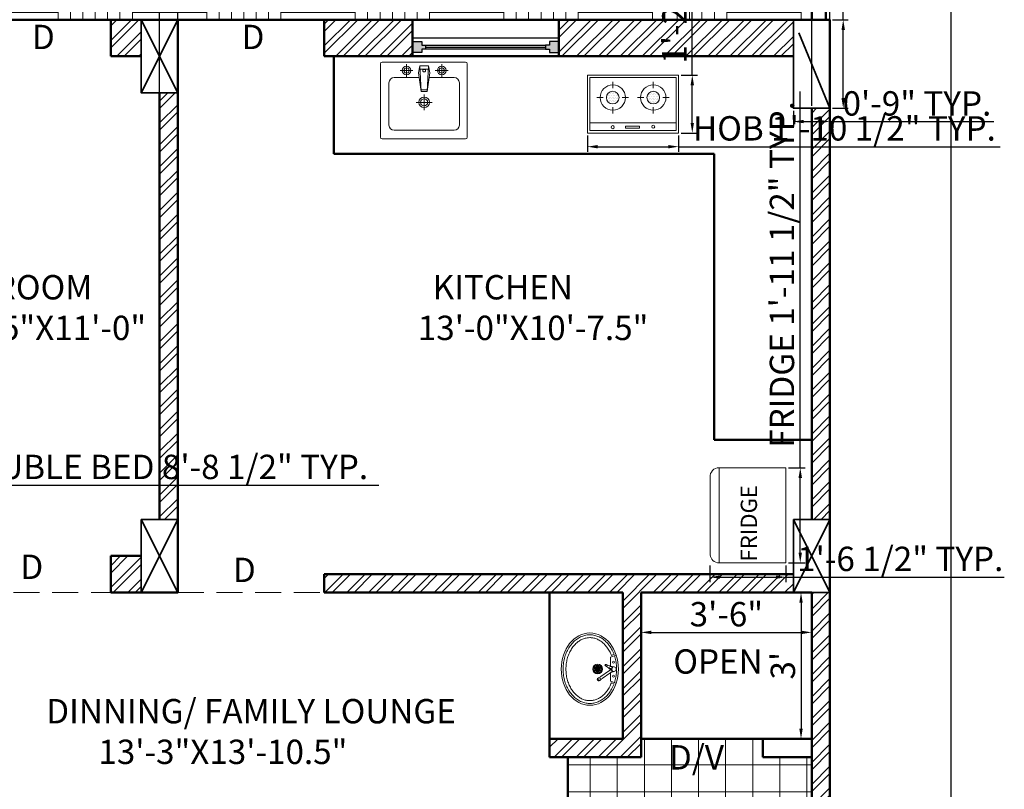
# Model space of a CAD drawing. Units: millimetres. Extents: x 67033 to 68301, y 155969 to 157209.
# Tile 15 of 17: x 67638 to 67880, y 156894 to 157083. Entities that reach past the tile are written whole.
import ezdxf

# ---------------------------------------------------------------- set-up
doc = ezdxf.new("R2010")
doc.units = ezdxf.units.MM
doc.linetypes.add('HIDDEN', pattern=[9.525, 6.35, -3.175])
for name, color, linetype, lineweight in [('A-ANNO-DIMS', 2, 'Continuous', 18), ('A-ANNO-TEXT', 7, 'Continuous', 18), ('A-AREA-IDEN', 3, 'Continuous', 18), ('A-COLS', 3, 'Continuous', 35), ('A-EQPM', 8, 'Continuous', 18), ('A-FLOR-FIXT', 9, 'Continuous', 18), ('A-FLOR-OVHD', 1, 'HIDDEN', 18), ('A-FLOR-PATT', 252, 'Continuous', 13), ('A-GLAZ', 4, 'Continuous', 25), ('A-WALL', 7, 'Continuous', 50), ('A-WALL-PATT', 8, 'Continuous', 13)]:
    doc.layers.add(name, color=color, linetype=linetype, lineweight=lineweight)
doc.styles.get("Standard").update_dxf_attribs({"font": 'arial.ttf'})
doc.dimstyles.new('ISO-25', dxfattribs={"dimtxt": 6, "dimasz": 2.5, "dimexe": 1.25, "dimexo": 0.625, "dimtad": 1, "dimdec": 0, "dimlunit": 3, "dimtxsty": 'Standard', "dimcen": 2.5, "dimadec": 0, "dimazin": 0, "dimtfac": 1, "dimtdec": 0, "dimtmove": 0, "dimatfit": 3, "dimfxl": 1, "dimarcsym": 0})
pattern_1 = [(45, (429.8785, 0), (-2.69407684, 2.69407684), []), (45, (431.6745, 0), (-2.69407684, 2.69407684), [])]

# ---------------------------------------------------------------- blocks, each defined once
blk = doc.blocks.new('A$C635F4E63')
for p, q in [((0, 10), (0, 426.6)), ((10, 436.6), (483.9, 436.6)), ((148.5, 425.2), (148.5, 352.2)), ((223.5, 415), (217, 376.2)), ((223.5, 415), (248.5, 415)), ((223.5, 415), (231.8, 268.5)), ((224.6, 395.4), (248.5, 395.4)), ((273.5, 415), (248.5, 415)), ((272.3, 395.4), (248.5, 395.4)), ((273.5, 415), (265.2, 268.5)), ((273.5, 415), (279.9, 376.2)), ((348.5, 425.2), (348.5, 352.2)), ((493.9, 426.6), (493.9, 10)), ((220.8, 348.8), (78.5, 348.8)), ((111.9, 388.7), (185, 388.7)), ((217, 376.2), (231.8, 268.5)), ((279.9, 376.2), (265.2, 268.5)), ((418.5, 348.8), (276.2, 348.8)), ((311.9, 388.7), (385, 388.7)), ((48.5, 318.8), (48.5, 78.8)), ((448.5, 318.8), (448.5, 78.8)), ((231.3, 278.6), (248.5, 278.6)), ((231.8, 268.5), (248.5, 268.5)), ((265.6, 278.6), (248.5, 278.6)), ((265.2, 268.5), (248.5, 268.5)), ((248.5, 252.8), (248.5, 162.6)), ((203.4, 207.7), (293.5, 207.7)), ((418.5, 48.8), (78.5, 48.8)), ((483.9, 0), (10, 0))]:
    blk.add_line(p, q)
for centre, radius in [((148.5, 388.7), 25), ((148.5, 388.7), 15), ((348.5, 388.7), 25), ((348.5, 388.7), 15), ((248.5, 207.7), 30), ((248.5, 207.7), 20)]:
    blk.add_circle(centre, radius)
for centre, radius, start, end in [((10, 426.6), 10, 90, 180), ((247.3, 388), 7.19, 80.5252, 279.4748), ((249.6, 388), 7.19, 260.5252, 99.4748), ((483.9, 426.6), 10, 0, 90), ((78.5, 318.8), 30, 90, 180), ((418.5, 318.8), 30, 0, 90), ((78.5, 78.8), 30, 180, 270), ((418.5, 78.8), 30, 270, 0), ((10, 10), 10, 180, 270), ((483.9, 10), 10, 270, 0)]:
    blk.add_arc(centre, radius, start, end)
blk = doc.blocks.new('A$C475E21CF')
for p, q in [((0, 444.5), (0, 0)), ((0, 444.5), (699.9, 444.5)), ((19.4, 425), (19.4, 19.4)), ((19.4, 425), (680.5, 425)), ((194.5, 393.9), (194.5, 345.2)), ((505.4, 393.9), (505.4, 345.2)), ((680.5, 425), (680.5, 19.4)), ((699.9, 444.5), (699.9, 0)), ((185.2, 312.7), (185.2, 312.7)), ((197.3, 312.7), (197.3, 312.7)), ((209.5, 312.7), (209.5, 312.7)), ((480.2, 304.5), (480.2, 304.5)), ((492.3, 304.5), (492.3, 304.5)), ((498.4, 316.6), (498.4, 316.6)), ((504.5, 304.5), (504.5, 304.5)), ((510.6, 316.6), (510.6, 316.6)), ((516.7, 304.5), (516.7, 304.5)), ((522.7, 316.6), (522.7, 316.6)), ((528.8, 304.5), (528.8, 304.5)), ((541, 304.5), (541, 304.5)), ((72.9, 272.3), (121.6, 272.3)), ((148.7, 264.1), (148.7, 264.1)), ((154.8, 276.2), (154.8, 276.2)), ((154.8, 251.9), (154.8, 251.9)), ((160.9, 288.4), (160.9, 288.4)), ((160.9, 264.1), (160.9, 264.1)), ((160.9, 239.8), (160.9, 239.8)), ((166.9, 300.5), (166.9, 300.5)), ((166.9, 276.2), (166.9, 276.2)), ((166.9, 251.9), (166.9, 251.9)), ((173, 288.4), (173, 288.4)), ((173, 264.1), (173, 264.1)), ((173, 239.8), (173, 239.8)), ((179.1, 300.5), (179.1, 300.5)), ((179.1, 276.2), (179.1, 276.2)), ((179.1, 251.9), (179.1, 251.9)), ((179.1, 227.6), (179.1, 227.6)), ((185.2, 288.4), (185.2, 288.4)), ((185.2, 264.1), (185.2, 264.1)), ((185.2, 239.8), (185.2, 239.8)), ((191.2, 300.5), (191.2, 300.5)), ((191.2, 276.2), (191.2, 276.2)), ((191.2, 251.9), (191.2, 251.9)), ((191.2, 227.6), (191.2, 227.6)), ((197.3, 288.4), (197.3, 288.4)), ((197.3, 264.1), (197.3, 264.1)), ((197.3, 239.8), (197.3, 239.8)), ((203.4, 300.5), (203.4, 300.5)), ((203.4, 276.2), (203.4, 276.2)), ((203.4, 251.9), (203.4, 251.9)), ((203.4, 227.6), (203.4, 227.6)), ((209.5, 288.4), (209.5, 288.4)), ((209.5, 264.1), (209.5, 264.1)), ((209.5, 239.8), (209.5, 239.8)), ((215.6, 300.5), (215.6, 300.5)), ((215.6, 276.2), (215.6, 276.2)), ((215.6, 251.9), (215.6, 251.9)), ((215.6, 227.6), (215.6, 227.6)), ((221.6, 288.4), (221.6, 288.4)), ((221.6, 264.1), (221.6, 264.1)), ((221.6, 239.8), (221.6, 239.8)), ((227.7, 300.5), (227.7, 300.5)), ((227.7, 276.2), (227.7, 276.2)), ((227.7, 251.9), (227.7, 251.9)), ((233.8, 288.4), (233.8, 288.4)), ((233.8, 264.1), (233.8, 264.1)), ((233.8, 239.8), (233.8, 239.8)), ((239.9, 276.2), (239.9, 276.2)), ((239.9, 251.9), (239.9, 251.9)), ((267.4, 272.3), (316, 272.3)), ((383.9, 272.3), (432.5, 272.3)), ((462, 268), (462, 268)), ((468, 280.2), (468, 280.2)), ((468, 255.9), (468, 255.9)), ((474.1, 292.3), (474.1, 292.3)), ((474.1, 268), (474.1, 268)), ((474.1, 243.7), (474.1, 243.7)), ((480.2, 280.2), (480.2, 280.2)), ((480.2, 255.9), (480.2, 255.9)), ((486.3, 292.3), (486.3, 292.3)), ((486.3, 268), (486.3, 268)), ((486.3, 243.7), (486.3, 243.7)), ((492.3, 280.2), (492.3, 280.2)), ((492.3, 255.9), (492.3, 255.9)), ((492.3, 231.5), (492.3, 231.5)), ((498.4, 292.3), (498.4, 292.3)), ((498.4, 268), (498.4, 268)), ((498.4, 243.7), (498.4, 243.7)), ((504.5, 280.2), (504.5, 280.2)), ((504.5, 255.9), (504.5, 255.9)), ((504.5, 231.5), (504.5, 231.5)), ((510.6, 292.3), (510.6, 292.3)), ((510.6, 268), (510.6, 268)), ((510.6, 243.7), (510.6, 243.7)), ((516.7, 280.2), (516.7, 280.2)), ((516.7, 255.9), (516.7, 255.9)), ((516.7, 231.5), (516.7, 231.5)), ((522.7, 292.3), (522.7, 292.3)), ((522.7, 268), (522.7, 268)), ((522.7, 243.7), (522.7, 243.7)), ((528.8, 280.2), (528.8, 280.2)), ((528.8, 255.9), (528.8, 255.9)), ((528.8, 231.5), (528.8, 231.5)), ((534.9, 292.3), (534.9, 292.3)), ((534.9, 268), (534.9, 268)), ((534.9, 243.7), (534.9, 243.7)), ((541, 280.2), (541, 280.2)), ((541, 255.9), (541, 255.9)), ((547, 292.3), (547, 292.3)), ((547, 268), (547, 268)), ((547, 243.7), (547, 243.7)), ((553.1, 280.2), (553.1, 280.2)), ((553.1, 255.9), (553.1, 255.9)), ((578.4, 272.3), (627, 272.3)), ((194.5, 199.4), (194.5, 150.8)), ((505.4, 199.4), (505.4, 150.8)), ((19.4, 77.8), (680.5, 77.8)), ((0, 0), (699.9, 0)), ((19.4, 19.4), (680.5, 19.4)), ((293.4, 51.9), (400.6, 51.9)), ((293.4, 36.5), (293.4, 51.9)), ((400.6, 36.5), (293.4, 36.5)), ((400.6, 51.9), (400.6, 36.5))]:
    blk.add_line(p, q)
for centre, radius in [((194.5, 272.3), 97.2), ((194.5, 272.3), 48.6), ((505.4, 272.3), 97.2), ((505.4, 272.3), 48.6), ((193.9, 45.1), 11.7), ((505.2, 48.5), 11.7)]:
    blk.add_circle(centre, radius)
blk = doc.blocks.new('A$C1AC47749')
for p, q in [((0.1857, 0.4482), (0.192, 0.4291)), ((0.1907, 0.471), (0.2068, 0.4222)), ((0.2068, 0.4222), (0.2842, 0.4222)), ((0.4132, 0.4222), (0.3413, 0.4222)), ((0.4293, 0.471), (0.4132, 0.4222)), ((0.4343, 0.4482), (0.428, 0.4291)), ((0.328, 0.4053), (0.3724, 0.3403)), ((0.3893, 0.3519), (0.3454, 0.4162))]:
    blk.add_line(p, q)
for centre, radius in [((0.2494, 0.448), 0.00831), ((0.3706, 0.448), 0.00831), ((0.3092, 0.3122), 0.0419), ((0.3092, 0.3122), 0.0344), ((0.3092, 0.3122), 0.00537)]:
    blk.add_circle(centre, radius)
for centre, radius, start, end in [((0.0375, 0.4868), 0.255, 336.13579, 352.27707), ((0.5085, 0.2596), 0.255, 136.21432, 152.3556), ((0.2063, 0.4499), 0.0866, 334.5047, 356.00596), ((0.31, 0.4499), 0.02, 316.21432, 172.27707), ((0.3092, 0.4498), 0.0162, 192.84427, 306.07085), ((0.3746, 0.3688), 0.0866, 132.48544, 153.98669), ((0.2456, 0.3486), 0.1, 34.51324, 47.88111), ((0.299, 0.3998), 0.0293, 33.00691, 56.74915), ((0.4278, 0.4728), 0.1, 191.02619, 214.5133), ((0.3603, 0.4414), 0.0293, 186.64626, 215.15328), ((0.2768, 0.381), 0.00664, 156.13579, 332.3556), ((0.2783, 0.3821), 0.00491, 187.76508, 270.74833), ((0.1778, 0.1242), 0.3257, 64.69826, 65.8021), ((0.29, 0.2836), 0.1, 20.01079, 34.51324), ((0.4717, 0.4086), 0.1, 214.5133, 229.01574), ((0.3971, 0.3226), 0.0139, 200.01079, 49.01574), ((0.3943, 0.3268), 0.00759, 93.32422, 152.57703), ((0.397, 0.323), 0.00812, 242.55567, 44.63645), ((0.3988, 0.322), 0.00965, 313.38275, 23.63796)]:
    blk.add_arc(centre, radius, start, end)
for centre, major_axis, ratio in [((0.31, 0.2449), (-0.31, 0), 0.790323), ((0.2993, 0.3294), (0.0072, -0.0126), 0.137964), ((0.3092, 0.332), (0, -0.0145), 0.137964), ((0.3192, 0.3294), (-0.0072, -0.0126), 0.137964), ((0.2894, 0.3122), (0.0145, 0), 0.137964), ((0.292, 0.3221), (0.0126, -0.0072), 0.137964), ((0.292, 0.3022), (0.0126, 0.0072), 0.137964), ((0.2993, 0.295), (0.0072, 0.0126), 0.137964), ((0.3092, 0.2923), (0, 0.0145), 0.137964), ((0.3192, 0.295), (-0.0072, 0.0126), 0.137964), ((0.3264, 0.3221), (-0.0126, -0.0072), 0.137964), ((0.3264, 0.3022), (-0.0126, 0.0072), 0.137964), ((0.3291, 0.3122), (-0.0145, 0), 0.137964)]:
    blk.add_ellipse(centre, major_axis=major_axis, ratio=ratio)
for points, knots in [([(0.1844, 0.4522), (0.1793, 0.4504), (0.1743, 0.4484), (0.1546, 0.44), (0.1406, 0.4328), (0.1143, 0.4165), (0.102, 0.4076), (0.0797, 0.3882), (0.0697, 0.3778), (0.052, 0.3558), (0.0443, 0.3443), (0.0317, 0.3205), (0.0267, 0.3083), (0.0194, 0.2833), (0.0171, 0.2706), (0.0158, 0.2536), (0.0156, 0.2492), (0.0156, 0.2449), (0.0156, 0.2369), (0.0162, 0.229), (0.019, 0.2084), (0.022, 0.1958), (0.0309, 0.1711), (0.0366, 0.159), (0.0508, 0.1357), (0.0591, 0.1244), (0.0781, 0.1031), (0.0888, 0.0931), (0.1123, 0.0746), (0.1251, 0.066), (0.1524, 0.0508), (0.1669, 0.0441), (0.1972, 0.0327), (0.213, 0.028), (0.2454, 0.0207), (0.262, 0.0182), (0.2956, 0.0154), (0.3125, 0.0152), (0.3462, 0.0169), (0.3629, 0.0189), (0.3956, 0.0251), (0.4117, 0.0293), (0.4426, 0.0397), (0.4574, 0.046), (0.4855, 0.0604), (0.4987, 0.0685), (0.5232, 0.0863), (0.5344, 0.096), (0.5545, 0.1167), (0.5635, 0.1277), (0.5788, 0.1506), (0.5851, 0.1625), (0.5953, 0.187), (0.599, 0.1995), (0.6037, 0.2248), (0.6047, 0.2375), (0.6039, 0.263), (0.6021, 0.2758), (0.5959, 0.3009), (0.5914, 0.3133), (0.5798, 0.3373), (0.5727, 0.349), (0.556, 0.3714), (0.5464, 0.382), (0.5249, 0.402), (0.5131, 0.4113), (0.4875, 0.4282), (0.4738, 0.4358), (0.4516, 0.446), (0.4437, 0.4492), (0.4356, 0.4522)], [5.14883, 5.14883, 5.14883, 5.14883, 5.205467, 5.205467, 5.375452, 5.375452, 5.545437, 5.545437, 5.715422, 5.715422, 5.885408, 5.885408, 6.055393, 6.055393, 6.225378, 6.225378, 6.283185, 6.283185, 6.283185, 6.389094, 6.389094, 6.559079, 6.559079, 6.729064, 6.729064, 6.89905, 6.89905, 7.069035, 7.069035, 7.23902, 7.23902, 7.409005, 7.409005, 7.578991, 7.578991, 7.748976, 7.748976, 7.918961, 7.918961, 8.088947, 8.088947, 8.258932, 8.258932, 8.428917, 8.428917, 8.598902, 8.598902, 8.768888, 8.768888, 8.938873, 8.938873, 9.108858, 9.108858, 9.278843, 9.278843, 9.448829, 9.448829, 9.618814, 9.618814, 9.788799, 9.788799, 9.958784, 9.958784, 10.12877, 10.12877, 10.298755, 10.298755, 10.46874, 10.46874, 10.559126, 10.559126, 10.559126, 10.559126]), ([(0.192, 0.4291), (0.1828, 0.4257), (0.1739, 0.4219), (0.1529, 0.4117), (0.1412, 0.4049), (0.1193, 0.3901), (0.1093, 0.382), (0.0911, 0.3649), (0.0829, 0.3558), (0.0687, 0.3371), (0.0626, 0.3273), (0.0526, 0.3074), (0.0487, 0.2972), (0.043, 0.2767), (0.0411, 0.2663), (0.0401, 0.2522), (0.04, 0.2486), (0.04, 0.2449), (0.04, 0.2369), (0.0406, 0.229), (0.0435, 0.2107), (0.0461, 0.2004), (0.0536, 0.1801), (0.0584, 0.1701), (0.0702, 0.1506), (0.0771, 0.1411), (0.093, 0.1229), (0.1019, 0.1142), (0.1217, 0.098), (0.1324, 0.0904), (0.1556, 0.0766), (0.168, 0.0704), (0.1939, 0.0596), (0.2075, 0.055), (0.2356, 0.0476), (0.2501, 0.0447), (0.2794, 0.0409), (0.2943, 0.0399), (0.3242, 0.0398), (0.3391, 0.0408), (0.3685, 0.0445), (0.3829, 0.0472), (0.4111, 0.0546), (0.4247, 0.0591), (0.4508, 0.0698), (0.4632, 0.076), (0.4864, 0.0897), (0.4973, 0.0972), (0.5171, 0.1134), (0.5262, 0.122), (0.5422, 0.1401), (0.5492, 0.1496), (0.561, 0.1691), (0.5659, 0.1791), (0.5736, 0.1994), (0.5763, 0.2097), (0.5797, 0.2304), (0.5803, 0.2408), (0.5794, 0.2617), (0.5779, 0.272), (0.5728, 0.2926), (0.5692, 0.3029), (0.5599, 0.3229), (0.5541, 0.3327), (0.5405, 0.3517), (0.5327, 0.3609), (0.5151, 0.3783), (0.5053, 0.3865), (0.4839, 0.4017), (0.4724, 0.4087), (0.4499, 0.4202), (0.4392, 0.4249), (0.428, 0.4291)], [5.15203, 5.15203, 5.15203, 5.15203, 5.262547, 5.262547, 5.423175, 5.423175, 5.583803, 5.583803, 5.744431, 5.744431, 5.90506, 5.90506, 6.065688, 6.065688, 6.226316, 6.226316, 6.283185, 6.283185, 6.283185, 6.405631, 6.405631, 6.566259, 6.566259, 6.726887, 6.726887, 6.887515, 6.887515, 7.048143, 7.048143, 7.208772, 7.208772, 7.3694, 7.3694, 7.530028, 7.530028, 7.690656, 7.690656, 7.851284, 7.851284, 8.011912, 8.011912, 8.172541, 8.172541, 8.333169, 8.333169, 8.493797, 8.493797, 8.654425, 8.654425, 8.815053, 8.815053, 8.975681, 8.975681, 9.13631, 9.13631, 9.296938, 9.296938, 9.457566, 9.457566, 9.618194, 9.618194, 9.778822, 9.778822, 9.93945, 9.93945, 10.100079, 10.100079, 10.260707, 10.260707, 10.421335, 10.421335, 10.555929, 10.555929, 10.555929, 10.555929]), ([(0.4244, 0.4561), (0.4209, 0.4573), (0.4174, 0.4584), (0.3981, 0.4641), (0.3818, 0.4677), (0.3487, 0.4726), (0.3319, 0.474), (0.2982, 0.4744), (0.2813, 0.4735), (0.248, 0.4694), (0.2315, 0.4663), (0.2088, 0.4603), (0.2022, 0.4583), (0.1956, 0.4561)], [4.3173628, 4.3173628, 4.3173628, 4.3173628, 4.3555402, 4.3555402, 4.5255255, 4.5255255, 4.6955107, 4.6955107, 4.865496, 4.865496, 5.0354813, 5.0354813, 5.1074083, 5.1074083, 5.1074083, 5.1074083])]:
    blk.add_open_spline(points, degree=3, knots=knots)
blk = doc.blocks.new('*D34')
at = {"layer": 'A-ANNO-DIMS', "color": 0, "lineweight": -2, "transparency": 16777216}
for p, q in [((67790.82, 156935.93), (67790.82, 156930.94)), ((67832.82, 156935.93), (67832.82, 156930.94)), ((67793.32, 156932.19), (67830.32, 156932.19))]:
    blk.add_line(p, q, dxfattribs=at)
at = {"layer": 'A-ANNO-DIMS', "color": 0, "transparency": 16777216}
for points in [[(67793.32, 156932.6), (67793.32, 156931.77), (67790.82, 156932.19)], [(67830.32, 156932.6), (67830.32, 156931.77), (67832.82, 156932.19)]]:
    blk.add_solid(points, dxfattribs=at)
at = {"layer": 'Defpoints', "color": 0, "transparency": 16777216}
for p in [(67790.82, 156936.55), (67832.82, 156936.55), (67832.82, 156932.19)]:
    blk.add_point(p, dxfattribs=at)
at = {"layer": 'A-ANNO-DIMS', "color": 0, "transparency": 16777216, "insert": (67811.82, 156935.88), "char_height": 6, "attachment_point": 5}
blk.add_mtext('3\'-6"', dxfattribs=at)
blk = doc.blocks.new('*D32')
at = {"layer": 'A-ANNO-DIMS', "color": 0, "lineweight": -2, "transparency": 16777216}
for p, q in [((67827.32, 156941.99), (67831.45, 156941.99)), ((67830.2, 156939.49), (67830.2, 156908.49)), ((67827.32, 156905.99), (67831.45, 156905.99))]:
    blk.add_line(p, q, dxfattribs=at)
at = {"layer": 'A-ANNO-DIMS', "color": 0, "transparency": 16777216}
for points in [[(67829.78, 156939.49), (67830.62, 156939.49), (67830.2, 156941.99)], [(67829.78, 156908.49), (67830.62, 156908.49), (67830.2, 156905.99)]]:
    blk.add_solid(points, dxfattribs=at)
at = {"layer": 'Defpoints', "color": 0, "transparency": 16777216}
for p in [(67826.69, 156941.99), (67826.69, 156905.99), (67830.2, 156905.99)]:
    blk.add_point(p, dxfattribs=at)
at = {"layer": 'A-ANNO-DIMS', "color": 0, "transparency": 16777216, "insert": (67826.51, 156923.99), "char_height": 6, "attachment_point": 5, "rotation": 90}
blk.add_mtext("3'", dxfattribs=at)
blk = doc.blocks.new('WIN-900')
for p, q in [((3.67, 3.22), (33.2, 3.22)), ((3.67, 2.74), (33.2, 2.74)), ((33.2, 2.27), (3.67, 2.27))]:
    blk.add_line(p, q)
blk.add_lwpolyline([(0.44, 4.99), (36.44, 4.99), (36.44, 0.49), (0.44, 0.49)], close=True)
for points in [[(0.44, 4.09), (2.73, 4.09), (2.73, 3.22), (3.67, 3.22), (3.67, 2.27), (2.73, 2.27), (2.73, 1.4), (0.44, 1.4)], [(36.44, 4.09), (34.14, 4.09), (34.14, 3.22), (33.2, 3.22), (33.2, 2.27), (34.14, 2.27), (34.14, 1.4), (36.44, 1.4)]]:
    blk.add_lwpolyline(points)
blk = doc.blocks.new('COLUMN-230x460')
for p, q in [((0.44, 17.99), (9.44, -0.01)), ((9.44, 17.99), (0.44, -0.01))]:
    blk.add_line(p, q)
blk.add_lwpolyline([(0.44, 17.99), (9.44, 17.99), (9.44, -0.01), (0.44, -0.01)], close=True)
blk = doc.blocks.new('COLUMN-TERR')
for p, q in [((9.32, 21.99), (9.32, 1.87)), ((1.64, 18.8), (9.32, 0.19))]:
    blk.add_line(p, q)
blk.add_lwpolyline([(0.32, 21.99), (9.32, 21.99), (9.32, 0.19), (0.32, 0.19)], close=True)
blk = doc.blocks.new('FRIDGE')
for p, q in [((18.68, 23.4), (2.13, 23.4)), ((2.2, 23.4), (2.2, 0)), ((18.68, 0), (18.68, 23.4)), ((0.01, 21.05), (0.01, 1.99)), ((2.13, 0), (18.68, 0))]:
    blk.add_line(p, q)
for centre, start, end in [((2.17, 21.23), 89.0957, 184.6304), ((2.17, 2.17), 184.6304, 270.9043)]:
    blk.add_arc(centre, 2.17, start, end)
blk = doc.blocks.new('*D55')
at = {"layer": 'A-ANNO-DIMS', "color": 0, "lineweight": -2, "transparency": 16777216}
for p, q in [((67511.46, 156983.46), (67511.46, 156967.16)), ((67615.96, 156983.46), (67615.96, 156967.16)), ((67513.96, 156968.41), (67613.46, 156968.41)), ((67615.96, 156968.41), (67726.32, 156968.41))]:
    blk.add_line(p, q, dxfattribs=at)
at = {"layer": 'A-ANNO-DIMS', "color": 0, "transparency": 16777216}
for points in [[(67513.96, 156968.83), (67513.96, 156967.99), (67511.46, 156968.41)], [(67613.46, 156968.83), (67613.46, 156967.99), (67615.96, 156968.41)]]:
    blk.add_solid(points, dxfattribs=at)
at = {"layer": 'Defpoints', "color": 0, "transparency": 16777216}
for p in [(67511.46, 156984.08), (67615.96, 156984.08), (67615.96, 156968.41)]:
    blk.add_point(p, dxfattribs=at)
at = {"layer": 'A-ANNO-DIMS', "color": 0, "transparency": 16777216, "insert": (67672.39, 156972.14), "char_height": 6, "attachment_point": 5}
blk.add_mtext('DOUBLE BED 8\'-8 1/2" TYP.', dxfattribs=at)
blk = doc.blocks.new('*D63')
at = {"layer": 'A-ANNO-DIMS', "color": 0, "lineweight": -2, "transparency": 16777216}
for p, q in [((67777.63, 157054.48), (67777.63, 157050.49)), ((67800.07, 157054.48), (67800.07, 157050.49)), ((67780.13, 157051.74), (67797.57, 157051.74)), ((67800.07, 157051.74), (67879.2, 157051.74))]:
    blk.add_line(p, q, dxfattribs=at)
at = {"layer": 'A-ANNO-DIMS', "color": 0, "transparency": 16777216}
for points in [[(67780.13, 157052.15), (67780.13, 157051.32), (67777.63, 157051.74)], [(67797.57, 157052.15), (67797.57, 157051.32), (67800.07, 157051.74)]]:
    blk.add_solid(points, dxfattribs=at)
at = {"layer": 'Defpoints', "color": 0, "transparency": 16777216}
for p in [(67777.63, 157055.1), (67800.07, 157055.1), (67800.07, 157051.74)]:
    blk.add_point(p, dxfattribs=at)
at = {"layer": 'A-ANNO-DIMS', "color": 0, "transparency": 16777216, "insert": (67840.88, 157055.47), "char_height": 6, "attachment_point": 5}
blk.add_mtext('HOB 1\'-10 1/2" TYP.', dxfattribs=at)
blk = doc.blocks.new('*D64')
at = {"layer": 'A-ANNO-DIMS', "color": 0, "lineweight": -2, "transparency": 16777216}
for p, q in [((67803.43, 157069.35), (67803.43, 157109.11)), ((67800.69, 157069.35), (67804.68, 157069.35)), ((67803.43, 157057.6), (67803.43, 157066.85)), ((67800.69, 157055.1), (67804.68, 157055.1))]:
    blk.add_line(p, q, dxfattribs=at)
at = {"layer": 'A-ANNO-DIMS', "color": 0, "transparency": 16777216}
for points in [[(67803.01, 157066.85), (67803.85, 157066.85), (67803.43, 157069.35)], [(67803.01, 157057.6), (67803.85, 157057.6), (67803.43, 157055.1)]]:
    blk.add_solid(points, dxfattribs=at)
at = {"layer": 'Defpoints', "color": 0, "transparency": 16777216}
for p in [(67800.07, 157069.35), (67803.43, 157069.35), (67800.07, 157055.1)]:
    blk.add_point(p, dxfattribs=at)
at = {"layer": 'A-ANNO-DIMS', "color": 0, "transparency": 16777216, "insert": (67799.79, 157090.48), "char_height": 6, "attachment_point": 5, "rotation": 90}
blk.add_mtext('1\'-2" TYP.', dxfattribs=at)
blk = doc.blocks.new('*D69')
at = {"layer": 'A-ANNO-DIMS', "color": 0, "lineweight": -2, "transparency": 16777216}
for p, q in [((67840.59, 157082.99), (67840.59, 157209.16)), ((67837.94, 157082.99), (67841.84, 157082.99)), ((67840.59, 157063.69), (67840.59, 157080.49)), ((67837.94, 157061.19), (67841.84, 157061.19))]:
    blk.add_line(p, q, dxfattribs=at)
at = {"layer": 'A-ANNO-DIMS', "color": 0, "transparency": 16777216}
for points in [[(67840.17, 157080.49), (67841, 157080.49), (67840.59, 157082.99)], [(67840.17, 157063.69), (67841, 157063.69), (67840.59, 157061.19)]]:
    blk.add_solid(points, dxfattribs=at)
at = {"layer": 'Defpoints', "color": 0, "transparency": 16777216}
for p in [(67837.32, 157082.99), (67840.59, 157082.99), (67837.32, 157061.19)]:
    blk.add_point(p, dxfattribs=at)
at = {"layer": 'A-ANNO-DIMS', "color": 0, "transparency": 16777216, "insert": (67836.86, 157147.33), "char_height": 6, "attachment_point": 5, "rotation": 90}
blk.add_mtext('TERRACE COLUMN 1\'-10" TYP.', dxfattribs=at)
blk = doc.blocks.new('*D70')
at = {"layer": 'A-ANNO-DIMS', "color": 0, "lineweight": -2, "transparency": 16777216}
for p, q in [((67828.32, 157060.57), (67828.32, 157056.67)), ((67837.32, 157060.57), (67837.32, 157056.67)), ((67830.82, 157057.92), (67834.82, 157057.92)), ((67837.32, 157057.92), (67877.64, 157057.92))]:
    blk.add_line(p, q, dxfattribs=at)
at = {"layer": 'A-ANNO-DIMS', "color": 0, "transparency": 16777216}
for points in [[(67830.82, 157058.34), (67830.82, 157057.51), (67828.32, 157057.92)], [(67834.82, 157058.34), (67834.82, 157057.51), (67837.32, 157057.92)]]:
    blk.add_solid(points, dxfattribs=at)
at = {"layer": 'Defpoints', "color": 0, "transparency": 16777216}
for p in [(67828.32, 157061.19), (67837.32, 157061.19), (67837.32, 157057.92)]:
    blk.add_point(p, dxfattribs=at)
at = {"layer": 'A-ANNO-DIMS', "color": 0, "transparency": 16777216, "insert": (67858.73, 157061.61), "char_height": 6, "attachment_point": 5}
blk.add_mtext('0\'-9" TYP.', dxfattribs=at)
blk = doc.blocks.new('*D71')
at = {"layer": 'A-ANNO-DIMS', "color": 0, "lineweight": -2, "transparency": 16777216}
for p, q in [((67830.01, 156972.72), (67830.01, 157065.34)), ((67827.12, 156972.72), (67831.26, 156972.72)), ((67830.01, 156951.79), (67830.01, 156970.22)), ((67827.12, 156949.29), (67831.26, 156949.29))]:
    blk.add_line(p, q, dxfattribs=at)
at = {"layer": 'A-ANNO-DIMS', "color": 0, "transparency": 16777216}
for points in [[(67829.59, 156970.22), (67830.43, 156970.22), (67830.01, 156972.72)], [(67829.59, 156951.79), (67830.43, 156951.79), (67830.01, 156949.29)]]:
    blk.add_solid(points, dxfattribs=at)
at = {"layer": 'Defpoints', "color": 0, "transparency": 16777216}
for p in [(67826.5, 156972.72), (67830.01, 156972.72), (67826.5, 156949.29)]:
    blk.add_point(p, dxfattribs=at)
at = {"layer": 'A-ANNO-DIMS', "color": 0, "transparency": 16777216, "insert": (67826.28, 157020.28), "char_height": 6, "attachment_point": 5, "rotation": 90}
blk.add_mtext('FRIDGE 1\'-11 1/2" TYP.', dxfattribs=at)
blk = doc.blocks.new('*D72')
at = {"layer": 'A-ANNO-DIMS', "color": 0, "lineweight": -2, "transparency": 16777216}
for p, q in [((67807.78, 156948.67), (67807.78, 156944.53)), ((67826.5, 156948.67), (67826.5, 156944.53)), ((67810.28, 156945.78), (67824, 156945.78)), ((67826.5, 156945.78), (67880.24, 156945.78))]:
    blk.add_line(p, q, dxfattribs=at)
at = {"layer": 'A-ANNO-DIMS', "color": 0, "transparency": 16777216}
for points in [[(67810.28, 156946.19), (67810.28, 156945.36), (67807.78, 156945.78)], [(67824, 156946.19), (67824, 156945.36), (67826.5, 156945.78)]]:
    blk.add_solid(points, dxfattribs=at)
at = {"layer": 'Defpoints', "color": 0, "transparency": 16777216}
for p in [(67807.78, 156949.29), (67826.5, 156949.29), (67826.5, 156945.78)]:
    blk.add_point(p, dxfattribs=at)
at = {"layer": 'A-ANNO-DIMS', "color": 0, "transparency": 16777216, "insert": (67854.62, 156949.5), "char_height": 6, "attachment_point": 5}
blk.add_mtext('1\'-6 1/2" TYP.', dxfattribs=at)
blk = doc.blocks.new('*D112')
at = {"layer": 'A-ANNO-DIMS', "color": 0, "lineweight": -2, "transparency": 16777216}
for p, q in [((67601.44, 157144.49), (67868.32, 157144.49)), ((67867.07, 157141.99), (67867.07, 156564.99)), ((67768.94, 156562.49), (67868.32, 156562.49))]:
    blk.add_line(p, q, dxfattribs=at)
at = {"layer": 'A-ANNO-DIMS', "color": 0, "transparency": 16777216}
for points in [[(67866.65, 157141.99), (67867.48, 157141.99), (67867.07, 157144.49)], [(67866.65, 156564.99), (67867.48, 156564.99), (67867.07, 156562.49)]]:
    blk.add_solid(points, dxfattribs=at)
at = {"layer": 'Defpoints', "color": 0, "transparency": 16777216}
for p in [(67600.82, 157144.49), (67768.32, 156562.49), (67867.07, 156562.49)]:
    blk.add_point(p, dxfattribs=at)
at = {"layer": 'A-ANNO-DIMS', "color": 0, "transparency": 16777216, "insert": (67863.38, 156853.49), "char_height": 6, "attachment_point": 5, "rotation": 90}
blk.add_mtext('48\'-6"', dxfattribs=at)
blk = doc.blocks.new('*D115')
at = {"layer": 'A-ANNO-DIMS', "color": 0, "lineweight": -2, "transparency": 16777216}
for p, q in [((67669.82, 157175.24), (67667.32, 157175.24)), ((67672.32, 156960.62), (67672.32, 157176.49)), ((67672.32, 157175.24), (67676.82, 157175.24)), ((67676.82, 156960.62), (67676.82, 157176.49)), ((67679.32, 157175.24), (67713, 157175.24))]:
    blk.add_line(p, q, dxfattribs=at)
at = {"layer": 'A-ANNO-DIMS', "color": 0, "transparency": 16777216}
for points in [[(67669.82, 157175.66), (67669.82, 157174.83), (67672.32, 157175.24)], [(67679.32, 157175.66), (67679.32, 157174.83), (67676.82, 157175.24)]]:
    blk.add_solid(points, dxfattribs=at)
at = {"layer": 'Defpoints', "color": 0, "transparency": 16777216}
for p in [(67676.82, 157175.24), (67672.32, 156959.99), (67676.82, 156959.99)]:
    blk.add_point(p, dxfattribs=at)
at = {"layer": 'A-ANNO-DIMS', "color": 0, "transparency": 16777216, "insert": (67697.41, 157178.97), "char_height": 6, "attachment_point": 5}
blk.add_mtext('0\'-4 1/2"', dxfattribs=at)
blk = doc.blocks.new('*D116')
at = {"layer": 'A-ANNO-DIMS', "color": 0, "lineweight": -2, "transparency": 16777216}
for p, q in [((67830.32, 157175.24), (67827.82, 157175.24)), ((67832.82, 157061.82), (67832.82, 157176.49)), ((67832.82, 157175.24), (67837.32, 157175.24)), ((67837.32, 157061.82), (67837.32, 157176.49)), ((67839.82, 157175.24), (67873.5, 157175.24))]:
    blk.add_line(p, q, dxfattribs=at)
at = {"layer": 'A-ANNO-DIMS', "color": 0, "transparency": 16777216}
for points in [[(67830.32, 157175.66), (67830.32, 157174.83), (67832.82, 157175.24)], [(67839.82, 157175.66), (67839.82, 157174.83), (67837.32, 157175.24)]]:
    blk.add_solid(points, dxfattribs=at)
at = {"layer": 'Defpoints', "color": 0, "transparency": 16777216}
for p in [(67837.32, 157175.24), (67832.82, 157061.19), (67837.32, 157061.19)]:
    blk.add_point(p, dxfattribs=at)
at = {"layer": 'A-ANNO-DIMS', "color": 0, "transparency": 16777216, "insert": (67857.91, 157178.97), "char_height": 6, "attachment_point": 5}
blk.add_mtext('0\'-4 1/2"', dxfattribs=at)

msp = doc.modelspace()

# ---------------------------------------------------------------- hatches: boundary and pattern name
at = {"layer": 'A-FLOR-PATT'}
h = msp.add_hatch(dxfattribs=at)
h.set_pattern_fill('AR-PARQ1', color=256, scale=0.06)
h.paths.add_polyline_path([(67832.82, 157112.99), (67597.32, 157112.99), (67597.32, 157140.99), (67567.32, 157140.99), (67567.32, 157082.99), (67627.32, 157082.99), (67660.32, 157082.99), (67832.82, 157082.99)])
h.paths.add_polyline_path([(67595.94, 157081.09), (67613.84, 157081.09), (67613.84, 157093.46), (67595.94, 157093.46)], flags=9)
h.paths.add_polyline_path([(67740.95, 157081.83), (67758.84, 157081.83), (67758.84, 157094.2), (67740.95, 157094.2)], flags=9)
h = msp.add_hatch(dxfattribs=at)
h.set_pattern_fill('NET', color=256, scale=2.1)
h.set_pattern_definition([(0, (429.8785, 0), (0, 6.6675), []), (90, (429.8785, 0), (-6.6675, 4e-16), [])])
h.paths.add_polyline_path([(67832.82, 156901.49), (67820.82, 156901.49), (67820.82, 156905.99), (67790.82, 156905.99), (67790.82, 156901.49), (67772.82, 156901.49), (67772.82, 156871.49), (67772.82, 156822.09), (67799.66, 156822.09), (67799.66, 156802.49), (67832.82, 156802.49)])
h.paths.add_polyline_path([(67823.43, 156839.69), (67824.62, 156840.78), (67832.57, 156840.81), (67832.57, 156830.35), (67832.57, 156819.92), (67824.62, 156819.92), (67823.54, 156820.91), (67809.23, 156822.7), (67807.41, 156823.26), (67805.06, 156824.94), (67803.4, 156827.36), (67802.63, 156830.25), (67803.17, 156832.59), (67804.67, 156835.13), (67806.89, 156836.98), (67809.3, 156837.81)], flags=16)
h.paths.add_polyline_path([(67813.05, 156836.69, -0.07076), (67816.48, 156836.17, -0.082382), (67819.17, 156834.8, -0.106831), (67821.11, 156832.58, -0.13423), (67821.71, 156830.24, -0.13423), (67821.11, 156827.91, -0.106831), (67819.17, 156825.68, -0.082382), (67816.48, 156824.32, -0.07076), (67813.05, 156823.8, -0.07076), (67809.61, 156824.32, -0.082382), (67806.92, 156825.68, -0.106831), (67804.99, 156827.91, -0.13423), (67804.39, 156830.24, -0.13423), (67804.99, 156832.58, -0.106831), (67806.92, 156834.8, -0.082382), (67809.61, 156836.17, -0.07076)], flags=0)
h.paths.add_polyline_path([(67823.39, 156830.38), (67823.43, 156830.25), (67823.38, 156830.35)], flags=0)
h.paths.add_polyline_path([(67824.5, 156840.03), (67824.49, 156840.02), (67823.96, 156839.53), (67824.95, 156836.55), (67824.94, 156833.37), (67823.92, 156830.35), (67824.94, 156827.34), (67824.95, 156824.16), (67823.96, 156821.17), (67824.49, 156820.68), (67824.75, 156820.52), (67825.04, 156820.46), (67825.05, 156820.46), (67825.04, 156820.46), (67824.75, 156820.52), (67824.49, 156820.68), (67823.96, 156821.17), (67824.95, 156824.16), (67824.94, 156827.34), (67823.92, 156830.35), (67824.94, 156833.37), (67824.95, 156836.55), (67823.96, 156839.53), (67824.5, 156840.03)], flags=0)
h.paths.add_polyline_path([(67826.5, 156838.81), (67831.02, 156838.81), (67831.02, 156830.35), (67831.02, 156821.89), (67826.5, 156821.89), (67826.17, 156822.61), (67826.61, 156826.35), (67825.85, 156830.02), (67825.72, 156830.35), (67826.59, 156834), (67826.26, 156837.75), (67826.17, 156838.09)], flags=0)
h.paths.add_polyline_path([(67820.79, 156830.25, -1), (67818.94, 156830.25, -1)], flags=0)
h.paths.add_polyline_path([(67792.51, 156895.05), (67814.14, 156895.05), (67814.14, 156907.42), (67792.51, 156907.42)], flags=9)
h.paths.add_polyline_path([(67782.63, 156854.97), (67824.6, 156854.97), (67824.6, 156877.36), (67782.63, 156877.36)], flags=24)
at = {"layer": 'A-GLAZ'}
h = msp.add_hatch(color=256, dxfattribs=at)
h.dxf.hatch_style = 1
h.paths.add_polyline_path([(67737.8, 157076.72), (67736.86, 157076.72), (67736.86, 157077.59), (67734.57, 157077.59), (67734.57, 157074.9), (67736.86, 157074.9), (67736.86, 157075.77), (67737.8, 157075.77)])
h = msp.add_hatch(color=256, dxfattribs=at)
h.dxf.hatch_style = 1
h.paths.add_polyline_path([(67770.57, 157077.59), (67768.27, 157077.59), (67768.27, 157076.72), (67767.33, 157076.72), (67767.33, 157075.77), (67768.27, 157075.77), (67768.27, 157074.9), (67770.57, 157074.9)])
at = {"layer": 'A-WALL-PATT'}
h = msp.add_hatch(dxfattribs=at)
h.set_pattern_fill('ANSI32', color=256, scale=0.4)
h.set_pattern_definition(pattern_1)
h.paths.add_polyline_path([(67667.82, 157082.99), (67660.32, 157082.99), (67660.32, 157073.99), (67667.82, 157073.99)])
h = msp.add_hatch(dxfattribs=at)
h.set_pattern_fill('ANSI32', color=256, scale=0.4)
h.set_pattern_definition(pattern_1)
h.paths.add_polyline_path([(67734.57, 157082.99), (67712.82, 157082.99), (67712.82, 157073.99), (67734.57, 157073.99)])
h = msp.add_hatch(dxfattribs=at)
h.set_pattern_fill('ANSI32', color=256, scale=0.4)
h.set_pattern_definition(pattern_1)
h.paths.add_polyline_path([(67828.32, 157082.99), (67770.57, 157082.99), (67770.57, 157073.99), (67828.32, 157073.99)])
h = msp.add_hatch(dxfattribs=at)
h.set_pattern_fill('ANSI32', color=256, scale=0.4)
h.set_pattern_definition(pattern_1)
h.paths.add_polyline_path([(67676.82, 157064.99), (67672.32, 157064.99), (67672.32, 156959.99), (67676.82, 156959.99)])
h = msp.add_hatch(dxfattribs=at)
h.set_pattern_fill('ANSI32', color=256, scale=0.4)
h.set_pattern_definition(pattern_1)
h.paths.add_polyline_path([(67837.32, 157061.19), (67832.82, 157061.19), (67832.82, 156959.99), (67837.32, 156959.99)])
h = msp.add_hatch(dxfattribs=at)
h.set_pattern_fill('ANSI32', color=256, scale=0.4)
h.set_pattern_definition(pattern_1)
h.paths.add_polyline_path([(67667.82, 156950.99), (67660.32, 156950.99), (67660.32, 156941.99), (67667.82, 156941.99)])
h = msp.add_hatch(dxfattribs=at)
h.set_pattern_fill('ANSI32', color=256, scale=0.4)
h.set_pattern_definition(pattern_1)
h.paths.add_polyline_path([(67828.32, 156946.49), (67712.82, 156946.49), (67712.82, 156941.99), (67786.32, 156941.99), (67786.32, 156905.99), (67768.32, 156905.99), (67768.32, 156901.49), (67790.82, 156901.49), (67790.82, 156941.99), (67828.32, 156941.99)])
h = msp.add_hatch(dxfattribs=at)
h.set_pattern_fill('ANSI32', color=256, scale=0.4)
h.set_pattern_definition(pattern_1)
h.paths.add_polyline_path([(67837.32, 156941.99), (67832.82, 156941.99), (67832.82, 156802.49), (67772.82, 156802.49), (67772.82, 156822.09), (67772.82, 156871.49), (67768.32, 156871.49), (67768.32, 156770.99), (67666.32, 156770.99), (67666.32, 156766.49), (67768.32, 156766.49), (67768.32, 156685.49), (67772.82, 156685.49), (67772.82, 156797.99), (67832.82, 156797.99), (67832.82, 156767.19), (67837.32, 156767.19)])

# ---------------------------------------------------------------- linework, layer by layer
at = {"layer": 'A-FLOR-OVHD'}
for p, q in [((67837.32, 157082.99), (67837.32, 157117.49)), ((67626.86, 156941.99), (67660.32, 156941.99)), ((67676.82, 156941.99), (67712.82, 156941.99))]:
    msp.add_line(p, q, dxfattribs=at)
at = {"layer": 'A-WALL'}
for p, q in [((67836.32, 157116.49), (67836.32, 157082.99)), ((67832.82, 157112.99), (67832.82, 157082.99)), ((67627.32, 157082.99), (67660.32, 157082.99)), ((67660.32, 157082.99), (67660.32, 157073.99)), ((67660.32, 157082.99), (67837.32, 157082.99)), ((67676.82, 157082.99), (67676.82, 156941.99)), ((67712.82, 157082.99), (67712.82, 157073.99)), ((67734.57, 157073.99), (67734.57, 157082.99)), ((67770.57, 157073.99), (67770.57, 157082.99)), ((67837.32, 157082.99), (67837.32, 156572.08)), ((67734.57, 157078.49), (67734.57, 157073.99)), ((67770.57, 157078.49), (67770.57, 157073.99)), ((67660.32, 157073.99), (67667.82, 157073.99)), ((67712.82, 157073.99), (67828.32, 157073.99)), ((67715.17, 157073.99), (67715.17, 157049.99)), ((67672.32, 157064.99), (67672.32, 156959.99)), ((67832.82, 157061.19), (67832.82, 156959.99)), ((67715.17, 157049.99), (67808.82, 157049.99)), ((67808.82, 157049.99), (67808.82, 156979.55)), ((67808.82, 156979.55), (67832.82, 156979.55)), ((67660.32, 156950.99), (67660.32, 156941.99)), ((67660.32, 156950.99), (67667.82, 156950.99)), ((67712.82, 156946.49), (67712.82, 156941.99)), ((67712.82, 156946.49), (67828.32, 156946.49)), ((67660.32, 156941.99), (67676.82, 156941.99)), ((67712.82, 156941.99), (67786.32, 156941.99)), ((67768.32, 156941.99), (67768.32, 156901.49)), ((67786.32, 156941.99), (67786.32, 156905.99)), ((67790.82, 156941.99), (67790.82, 156901.49)), ((67790.82, 156941.99), (67832.82, 156941.99)), ((67832.82, 156941.99), (67832.82, 156802.49)), ((67768.32, 156905.99), (67786.32, 156905.99)), ((67820.82, 156905.99), (67790.82, 156905.99)), ((67820.82, 156905.99), (67820.82, 156901.49)), ((67820.82, 156905.99), (67832.82, 156905.99)), ((67768.32, 156901.49), (67790.82, 156901.49)), ((67772.82, 156871.49), (67772.82, 156901.49)), ((67820.82, 156901.49), (67832.82, 156901.49))]:
    msp.add_line(p, q, dxfattribs=at)

# ---------------------------------------------------------------- block references
at = {"layer": 'A-COLS'}
for name, p in [('COLUMN-230x460', (67667.38, 157065)), ('COLUMN-TERR', (67828, 157061)), ('COLUMN-230x460', (67667.38, 156942)), ('COLUMN-230x460', (67827.88, 156942))]:
    msp.add_blockref(name, p, dxfattribs=at)
at = {"layer": 'A-EQPM'}
msp.add_blockref('FRIDGE', (67807.82, 156949.31), dxfattribs=at)
at = {"layer": 'A-FLOR-FIXT'}
for name, p, xscale, yscale, zscale in [('A$C635F4E63', (67726.67, 157053.65), 0.0433159964901652, 0.0433159964901652, 0.0433159964901652), ('A$C475E21CF', (67777.63, 157055.1), 0.0320579729999927, 0.0320579729999927, 0.0320579729999927)]:
    msp.add_blockref(name, p, dxfattribs=dict(at, xscale=xscale, yscale=yscale, zscale=zscale))
at = {"layer": 'A-FLOR-FIXT', "xscale": 28.71035709425155, "yscale": 28.71035709425155, "zscale": 28.71035709425155, "rotation": 270}
msp.add_blockref('A$C1AC47749', (67771.19, 156932.04), dxfattribs=at)
at = {"layer": 'A-GLAZ'}
msp.add_blockref('WIN-900', (67734.13, 157073.5), dxfattribs=at)

# ---------------------------------------------------------------- texts
at = {"layer": 'A-ANNO-TEXT', "char_height": 6, "attachment_point": 1}
for s, insert in [('   D', (67635.39, 157081.74)), ('   D', (67686.98, 157081.74)), ('   D', (67632.55, 156951.32)), ('   D', (67684.86, 156950.57)), ('  D/V', (67794.01, 156904.43))]:
    msp.add_mtext_dynamic_manual_height_columns(s, width=19.5287, gutter_width=12.5, heights=[0], dxfattribs=dict(at, insert=insert))
at = {"layer": 'A-ANNO-TEXT', "insert": (67815.36, 156945.96), "char_height": 4, "attachment_point": 1, "rotation": 90}
msp.add_mtext_dynamic_manual_height_columns('   FRIDGE', width=46.8836, gutter_width=12.5, heights=[0], dxfattribs=at)
at = {"layer": 'A-AREA-IDEN', "char_height": 6, "attachment_point": 1}
for s, width, insert in [('  BEDROOM \\P14\'-1.5"X11\'-0"', 59.4046, (67612.25, 157020.14)), ('  KITCHEN\\P13\'-0"X10\'-7.5"', 62.0967, (67735.87, 157020.14)), ('        OPEN', 46.8836, (67784.1, 156928.02)), ('  DINNING/ FAMILY LOUNGE\\P         13\'-3"X13\'-10.5"', 118.0294, (67640.74, 156915.79))]:
    msp.add_mtext_dynamic_manual_height_columns(s, width=width, gutter_width=12.5, heights=[0], dxfattribs=dict(at, insert=insert))

# ---------------------------------------------------------------- dimensions: what is measured, and where the dimension line sits
at = {"layer": 'A-ANNO-DIMS'}
for base, p1, p2, text, picture, middle in [((67840.59, 157082.99), (67837.32, 157061.19), (67837.32, 157082.99), 'TERRACE COLUMN <> TYP.', '*D69', (67836.86, 157147.33)), ((67803.431, 157069.3533), (67800.0652, 157055.1037), (67800.0652, 157069.3533), '<> TYP.', '*D64', (67799.7916, 157090.4824)), ((67830.01, 156972.72), (67826.5, 156949.29), (67826.5, 156972.72), 'FRIDGE <> TYP.', '*D71', (67826.28, 157020.28))]:
    dim = msp.add_linear_dim(base=base, p1=p1, p2=p2, angle=90, text=text, dimstyle='ISO-25', override={"dimdec": 1, "dimrnd": 0, "dimzin": 1, "dimlunit": 4, "dimfrac": 2}, dxfattribs=at)
    dim.commit()
    dim.dimension.update_dxf_attribs({"geometry": picture, "text_midpoint": middle})
for base, p1, p2, override, picture, middle in [((67676.82, 157175.24), (67672.32, 156959.99), (67676.82, 156959.99), {"dimdec": 1, "dimlfac": 1, "dimrnd": 0, "dimzin": 1, "dimdsep": 46, "dimlunit": 4, "dimfrac": 2}, '*D115', (67697.41, 157178.97)), ((67837.32, 157175.24), (67832.82, 157061.19), (67837.32, 157061.19), {"dimdec": 1, "dimlfac": 1, "dimrnd": 0, "dimzin": 1, "dimdsep": 46, "dimlunit": 4, "dimfrac": 2}, '*D116', (67857.91, 157178.97)), ((67832.82, 156932.19), (67790.82, 156936.55), (67832.82, 156936.55), {"dimclrd": 0, "dimclre": 0, "dimclrt": 0}, '*D34', (67811.82, 156935.88))]:
    dim = msp.add_linear_dim(base=base, p1=p1, p2=p2, dimstyle='ISO-25', override=override, dxfattribs=at)
    dim.commit()
    dim.dimension.update_dxf_attribs({"geometry": picture, "text_midpoint": middle})
for base, p1, p2, override, picture, middle in [((67867.07, 156562.49), (67600.82, 157144.49), (67768.32, 156562.49), {"dimdec": 1, "dimlfac": 1, "dimrnd": 0, "dimzin": 1, "dimdsep": 46, "dimlunit": 4, "dimfrac": 2}, '*D112', (67863.38, 156853.49)), ((67830.2, 156905.99), (67826.69, 156941.99), (67826.69, 156905.99), {"dimclrd": 0, "dimclre": 0, "dimclrt": 0}, '*D32', (67826.51, 156923.99))]:
    dim = msp.add_linear_dim(base=base, p1=p1, p2=p2, angle=90, dimstyle='ISO-25', override=override, dxfattribs=at)
    dim.commit()
    dim.dimension.update_dxf_attribs({"geometry": picture, "text_midpoint": middle})
for base, p1, p2, text, picture, middle in [((67800.07, 157051.74), (67777.63, 157055.1), (67800.07, 157055.1), 'HOB <> TYP.', '*D63', (67840.88, 157055.47)), ((67837.32, 157057.92), (67828.32, 157061.19), (67837.32, 157061.19), '<> TYP.', '*D70', (67858.73, 157061.61)), ((67615.96, 156968.41), (67511.46, 156984.08), (67615.96, 156984.08), 'DOUBLE BED <> TYP.', '*D55', (67672.39, 156972.14)), ((67826.5, 156945.78), (67807.78, 156949.29), (67826.5, 156949.29), '<> TYP.', '*D72', (67854.62, 156949.5))]:
    dim = msp.add_linear_dim(base=base, p1=p1, p2=p2, text=text, dimstyle='ISO-25', override={"dimdec": 1, "dimrnd": 0, "dimzin": 1, "dimlunit": 4, "dimfrac": 2}, dxfattribs=at)
    dim.commit()
    dim.dimension.update_dxf_attribs({"geometry": picture, "text_midpoint": middle})

doc.saveas('drawing.dxf')
